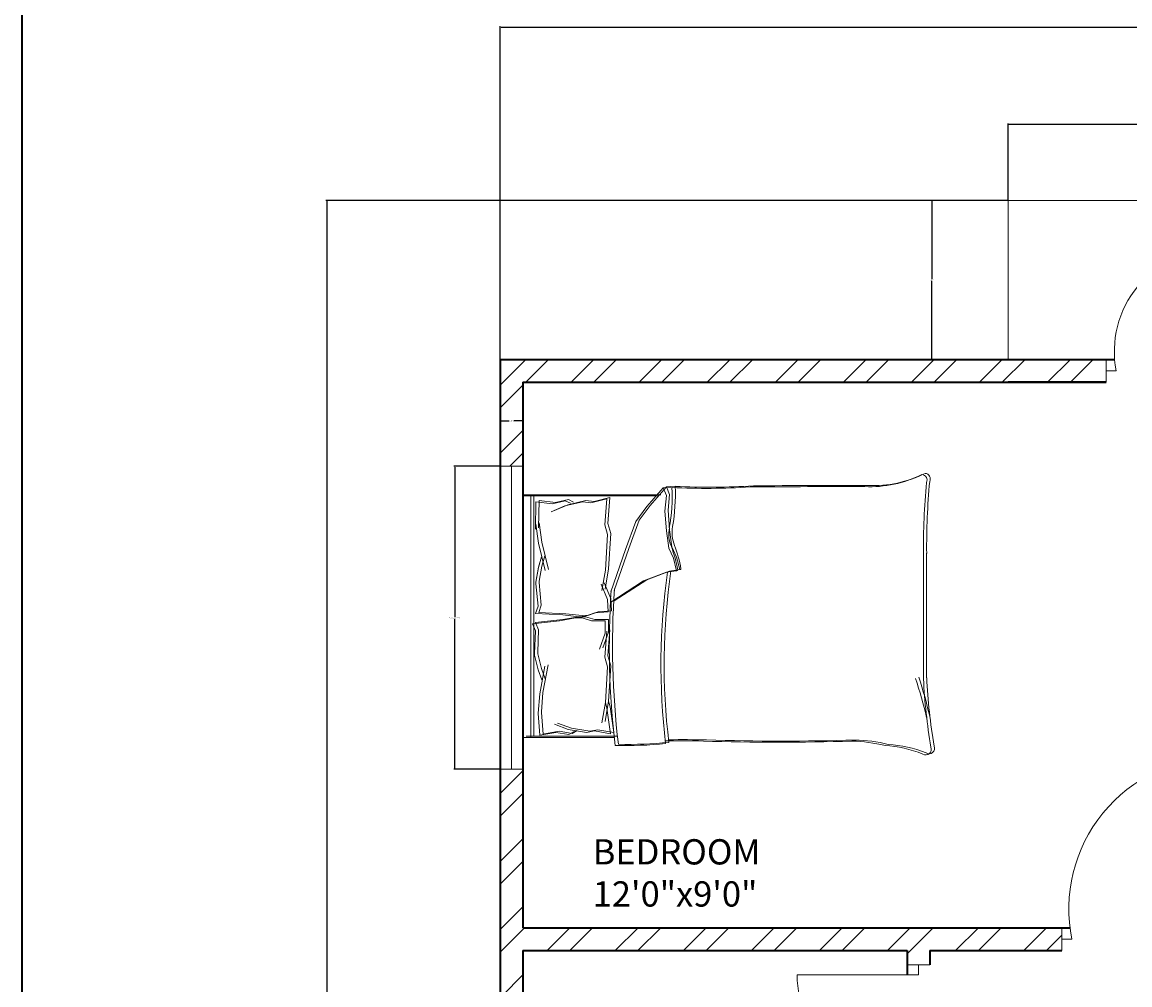
# Model space of a CAD drawing. Units: inches. Extents: x 2165 to 3042, y 1626 to 2968.
# Tile 3 of 11: x 2192 to 2411, y 2208 to 2399. Entities that reach past the tile are written whole.
import ezdxf

# ---------------------------------------------------------------- set-up
doc = ezdxf.new("R2010")
doc.units = ezdxf.units.IN
for name, color, linetype, lineweight in [('A-ANNO-DIMS', 2, 'Continuous', 18), ('A-AREA-IDEN', 7, 'Continuous', 18), ('A-DOOR', 3, 'Continuous', 18), ('A-FLOR-BALC', 7, 'Continuous', 18), ('A-FURN', 8, 'Continuous', 13), ('A-GLAZ', 4, 'Continuous', 18), ('A-WALL', 7, 'Continuous', 35), ('A-WALL-PATT', 252, 'Continuous', 13)]:
    doc.layers.add(name, color=color, linetype=linetype, lineweight=lineweight)
doc.styles.get("Standard").update_dxf_attribs({"font": 'arial.ttf'})
doc.dimstyles.get("Standard").update_dxf_attribs({"dimtxt": 0.18, "dimasz": 0.18, "dimexe": 0.18, "dimexo": 0.0625, "dimgap": 0.09, "dimtad": 0, "dimtih": 1, "dimtoh": 1, "dimdec": 4, "dimzin": 0, "dimdsep": 46, "dimtxsty": 'Standard', "dimcen": 0.09, "dimadec": 0, "dimazin": 0, "dimtfac": 1, "dimtdec": 4, "dimtofl": 0, "dimtmove": 0, "dimatfit": 3, "dimfxl": 1, "dimtolj": 1, "dimtzin": 0, "dimarcsym": 0})

# ---------------------------------------------------------------- blocks, each defined once
blk = doc.blocks.new('BED-DOUBLE')
for p, q in [((27.75, 52.87), (24.5, 49.16)), ((27.75, 52.87), (24.5, 49.16)), ((28.39, 53.1), (25.14, 49.39)), ((28.39, 53.1), (25.14, 49.39)), ((29.49, 52.95), (27.75, 52.87, 3.87)), ((29.49, 52.95), (27.75, 52.87, 3.87)), ((28.37, 51.33), (27.75, 52.87)), ((28.37, 51.33), (27.75, 52.87)), ((30.13, 53.18), (28.39, 53.1, 3.87)), ((30.13, 53.18), (28.39, 53.1, 3.87)), ((29, 51.56), (28.39, 53.1)), ((29, 51.56), (28.39, 53.1)), ((0, 51.27), (0, 51.49)), ((0, 51.49), (0.64, 51.49)), ((0, 51.27), (26.61, 51.27)), ((0, 51.27), (26.61, 51.27)), ((0, 51.27), (0, 3.48)), ((0.64, 51.49), (27.25, 51.49)), ((0.64, 51.49), (27.25, 51.49)), ((1.53, 3.48), (1.53, 51.27)), ((1.53, 3.47), (1.53, 51.27)), ((2.17, 3.7), (2.17, 51.49)), ((2.17, 3.7), (2.17, 51.49)), ((6.41, 49.96), (8.98, 50.56)), ((6.41, 49.96), (8.98, 50.56)), ((8.98, 50.56), (10.02, 50.04)), ((8.98, 50.56), (10.02, 50.04)), ((16.57, 50.7), (13.43, 49.92)), ((16.57, 50.7), (13.43, 49.92)), ((17.21, 50.93), (14.07, 50.15)), ((17.21, 50.93), (14.07, 50.15)), ((16.17, 45.57), (16.57, 50.7)), ((16.17, 45.57), (16.57, 50.7)), ((16.81, 45.79), (17.21, 50.93)), ((16.81, 45.79), (17.21, 50.93)), ((28.06, 48.23), (28.37, 51.33)), ((28.06, 48.23), (28.37, 51.33)), ((28.7, 48.46), (29, 51.56)), ((28.7, 48.46), (29, 51.56)), ((2.56, 50.11), (2.46, 44.71)), ((2.56, 50.11), (2.46, 44.71)), ((2.56, 50.11), (5.77, 49.73)), ((2.56, 50.11), (5.77, 49.73)), ((3.2, 50.34), (3.1, 44.94)), ((3.2, 50.34), (3.1, 44.94)), ((3.2, 50.34), (6.41, 49.96)), ((3.2, 50.34), (6.41, 49.96)), ((8.26, 49.31), (5.58, 48.13)), ((8.26, 49.31), (5.58, 48.13)), ((5.77, 49.73), (8.34, 50.33)), ((5.77, 49.73), (8.34, 50.33)), ((8.9, 49.54), (6.22, 48.36)), ((8.9, 49.54), (6.22, 48.36)), ((11.83, 50.11), (8.26, 49.31)), ((11.83, 50.11), (8.26, 49.31)), ((8.34, 50.33), (9.38, 49.81)), ((8.34, 50.33), (9.38, 49.81)), ((12.47, 50.34), (8.9, 49.54)), ((12.47, 50.34), (8.9, 49.54)), ((13.43, 49.92), (11.83, 50.11)), ((13.43, 49.92), (11.83, 50.11)), ((14.07, 50.15), (12.47, 50.34)), ((14.07, 50.15), (12.47, 50.34)), ((24.5, 49.16), (22.33, 46.22)), ((24.5, 49.16), (22.33, 46.22)), ((25.14, 49.39), (22.97, 46.45)), ((25.14, 49.39), (22.97, 46.45)), ((28.37, 44.36), (28.06, 48.23)), ((28.37, 44.36), (28.06, 48.23)), ((29, 44.59), (28.7, 48.46)), ((29, 44.59), (28.7, 48.46)), ((22.33, 46.22), (20.32, 40.64)), ((22.33, 46.22), (20.32, 40.64)), ((22.97, 46.45), (20.96, 40.87)), ((22.97, 46.45), (20.96, 40.87)), ((2.46, 44.71), (2.54, 45.71)), ((2.46, 44.71), (2.54, 45.71)), ((2.54, 45.71), (3.07, 41.91)), ((2.54, 45.71), (3.07, 41.91)), ((3.1, 44.94), (3.18, 45.94)), ((3.1, 44.94), (3.18, 45.94)), ((3.18, 45.94), (3.71, 42.14)), ((3.18, 45.94), (3.71, 42.14)), ((16.73, 43.61), (16.17, 45.57)), ((16.73, 43.61), (16.17, 45.57)), ((17.37, 43.83), (16.81, 45.79)), ((17.37, 43.83), (16.81, 45.79)), ((28.83, 40.95), (28.37, 44.36)), ((28.83, 40.95), (28.37, 44.36)), ((29.47, 41.18), (29, 44.59)), ((29.47, 41.18), (29, 44.59)), ((3.07, 41.91), (4.42, 36.5)), ((3.07, 41.91), (4.42, 36.49)), ((3.71, 42.14), (5.06, 36.72)), ((3.71, 42.14), (5.06, 36.72)), ((16.3, 36.6), (16.73, 43.61)), ((16.3, 36.6), (16.73, 43.61)), ((16.93, 36.82), (17.37, 43.83)), ((16.93, 36.82), (17.37, 43.83)), ((20.32, 40.64), (17.38, 32.31)), ((20.32, 40.64), (17.38, 32.31)), ((20.96, 40.87), (18.02, 32.53)), ((20.96, 40.87), (18.02, 32.53)), ((29.76, 38.94), (28.83, 40.95)), ((29.76, 38.94), (28.83, 40.95)), ((30.4, 39.17), (29.47, 41.18)), ((30.4, 39.17), (29.47, 41.18)), ((79.25, 15.06), (79.25, 39.68)), ((79.25, 15.06), (79.25, 39.68)), ((79.88, 15.29), (79.88, 39.91)), ((79.88, 15.29), (79.88, 39.91)), ((3.67, 39.2), (3.08, 37.14)), ((3.67, 39.2), (3.08, 37.13)), ((3.72, 37.36), (3.18, 34.43)), ((3.72, 37.36), (3.18, 34.43)), ((4.31, 39.43), (3.72, 37.36)), ((4.31, 39.43), (3.72, 37.36)), ((30.38, 36.46), (29.76, 38.94)), ((30.38, 36.46), (29.76, 38.94)), ((31.02, 36.69), (30.4, 39.17)), ((31.02, 36.69), (30.4, 39.17)), ((3.08, 37.14), (2.54, 34.2)), ((3.08, 37.13), (2.54, 34.2)), ((15.63, 32.56), (16.3, 36.6)), ((15.63, 32.56), (16.3, 36.6)), ((16.27, 32.79), (16.93, 36.82)), ((16.27, 32.79), (16.93, 36.82)), ((23.88, 34.45), (28.37, 36.15)), ((23.88, 34.45), (28.37, 36.15)), ((24.52, 34.68), (29, 36.38)), ((24.52, 34.68), (29, 36.38)), ((28.37, 36.15), (30.38, 36.46)), ((28.37, 36.15), (30.38, 36.46)), ((29, 36.38), (31.02, 36.69)), ((29, 36.38), (31.02, 36.69)), ((2.54, 34.2), (2.56, 33.88)), ((2.54, 34.2), (2.56, 33.88)), ((2.56, 33.88), (2.98, 29.46)), ((2.56, 33.88), (2.98, 29.46)), ((3.18, 34.43), (3.2, 34.11)), ((3.18, 34.43), (3.2, 34.11)), ((3.2, 34.11), (3.62, 29.68)), ((3.2, 34.11), (3.62, 29.68)), ((16.74, 30.75), (15.46, 33.82)), ((16.74, 30.75), (15.46, 33.82)), ((17.38, 30.98), (16.09, 34.05)), ((17.38, 30.98), (16.09, 34.05)), ((17.38, 30.26), (23.88, 34.45)), ((17.38, 30.26), (23.88, 34.45)), ((18.02, 30.49), (24.52, 34.68)), ((18.02, 30.49), (24.52, 34.68)), ((16.89, 28.3), (16.74, 30.75)), ((16.89, 28.3), (16.74, 30.75)), ((17.53, 28.53), (17.38, 30.98)), ((17.53, 28.53), (17.38, 30.98)), ((2.98, 29.46), (2.49, 27.98)), ((2.98, 29.46), (2.49, 27.98)), ((3.62, 29.68), (3.13, 28.21)), ((3.62, 29.68), (3.13, 28.21)), ((14.86, 28.36), (17.53, 28.53)), ((14.86, 28.36), (17.53, 28.53)), ((1.87, 25.98), (7.22, 26.56)), ((1.87, 25.98), (7.22, 26.56)), ((2.49, 27.98), (7.87, 27.73)), ((2.49, 27.98), (7.87, 27.73)), ((2.51, 26.21), (7.86, 26.79)), ((2.51, 26.21), (7.86, 26.79)), ((3.13, 28.21), (8.51, 27.96)), ((3.13, 28.21), (8.51, 27.96)), ((7.22, 26.56), (10.4, 27.14)), ((7.22, 26.56), (10.4, 27.14)), ((7.86, 26.79), (11.04, 27.37)), ((7.86, 26.79), (11.04, 27.37)), ((7.87, 27.73), (11.08, 27.35)), ((7.87, 27.73), (11.08, 27.35)), ((8.51, 27.96), (11.72, 27.58)), ((8.51, 27.96), (11.72, 27.58)), ((10.4, 27.14), (11.7, 27.14)), ((10.4, 27.14), (11.7, 27.14)), ((11.04, 27.37), (12.34, 27.37)), ((11.04, 27.37), (12.34, 27.37)), ((11.08, 27.35), (12.38, 27.44)), ((11.08, 27.35), (12.38, 27.44)), ((11.7, 27.14), (13.58, 26.56)), ((11.7, 27.14), (13.58, 26.56)), ((11.72, 27.58), (13.02, 27.66)), ((11.72, 27.58), (13.02, 27.66)), ((12.34, 27.37), (14.22, 26.79)), ((12.34, 27.37), (14.22, 26.79)), ((12.38, 27.44), (14.22, 28.13)), ((12.38, 27.44), (14.22, 28.13)), ((13.02, 27.66), (14.86, 28.36)), ((13.02, 27.66), (14.86, 28.36)), ((13.58, 26.56), (16.26, 26.56)), ((13.58, 26.56), (16.26, 26.56)), ((14.22, 28.13), (16.89, 28.3)), ((14.22, 28.13), (16.89, 28.3)), ((14.22, 26.79), (16.9, 26.79)), ((14.22, 26.79), (16.9, 26.79)), ((16.26, 26.56), (16.26, 24.1)), ((16.26, 26.56), (16.26, 24.1)), ((16.9, 26.79), (16.9, 24.33)), ((16.9, 26.79), (16.9, 24.33)), ((2.45, 24.54), (1.87, 25.98)), ((2.45, 24.54), (1.87, 25.98)), ((2.3, 20.09), (2.45, 24.54)), ((2.3, 20.09), (2.45, 24.54)), ((3.09, 24.77), (2.51, 26.21)), ((3.09, 24.77), (2.51, 26.21)), ((2.94, 20.32), (3.09, 24.77)), ((2.94, 20.32), (3.09, 24.77)), ((16.9, 24.33), (15.81, 21.19)), ((16.9, 24.33), (15.81, 21.19)), ((16.17, 19.38), (16.57, 24.52)), ((16.17, 19.38), (16.57, 24.52)), ((16.81, 19.61), (17.21, 24.74)), ((16.81, 19.61), (17.21, 24.74)), ((16.26, 24.1), (15.17, 20.96)), ((16.26, 24.1), (15.17, 20.96)), ((2.3, 19.77), (2.3, 20.09)), ((2.3, 19.77), (2.3, 20.09)), ((3.03, 16.88), (2.3, 19.77)), ((3.03, 16.88), (2.3, 19.77)), ((2.94, 20), (2.94, 20.32)), ((2.94, 20), (2.94, 20.32)), ((3.67, 17.11), (2.94, 20)), ((3.67, 17.11), (2.94, 20)), ((3.32, 12.11), (4.33, 17.6)), ((3.32, 12.11), (4.33, 17.6)), ((3.96, 12.34), (4.97, 17.83)), ((3.96, 12.34), (4.97, 17.83)), ((16.73, 17.42), (16.17, 19.38)), ((16.73, 17.42), (16.17, 19.38)), ((17.37, 17.65), (16.81, 19.61)), ((17.37, 17.65), (16.81, 19.61)), ((16.93, 10.64), (17.37, 17.65)), ((16.93, 10.64), (17.37, 17.65)), ((3.75, 14.85), (3.03, 16.88)), ((3.75, 14.85), (3.03, 16.88)), ((4.39, 15.08), (3.67, 17.11)), ((4.39, 15.08), (3.67, 17.11)), ((16.3, 10.41), (16.73, 17.42)), ((16.3, 10.41), (16.73, 17.42)), ((3.03, 8.28), (3.32, 12.11)), ((3.03, 8.28), (3.32, 12.11)), ((3.67, 8.51), (3.96, 12.34)), ((3.67, 8.51), (3.96, 12.34)), ((15.63, 6.38), (16.3, 10.41)), ((15.63, 6.38), (16.3, 10.41)), ((16.27, 6.61), (16.93, 10.64)), ((16.27, 6.61), (16.93, 10.64)), ((16.3, 10.41), (16.62, 9.28)), ((16.3, 10.41), (16.62, 9.28)), ((16.62, 9.28), (17.34, 4.18)), ((16.62, 9.28), (17.34, 4.18)), ((16.93, 10.64), (17.26, 9.51)), ((16.93, 10.64), (17.26, 9.51)), ((17.26, 9.51), (17.98, 4.41)), ((17.26, 9.51), (17.98, 4.41)), ((3.01, 8.18), (3.03, 8.28)), ((3.01, 8.18), (3.03, 8.28)), ((3.34, 3.9), (3.01, 8.18)), ((3.34, 3.9), (3.01, 8.18)), ((3.65, 8.41), (3.67, 8.51)), ((3.65, 8.41), (3.67, 8.51)), ((3.98, 4.13), (3.65, 8.41)), ((3.98, 4.13), (3.65, 8.41)), ((3.32, 3.89), (6.5, 4.47)), ((3.32, 3.89), (6.5, 4.47)), ((3.96, 4.12), (7.14, 4.7)), ((3.96, 4.12), (7.14, 4.7)), ((8.96, 5.05), (6.21, 6.06)), ((8.96, 5.05), (6.21, 6.06)), ((6.5, 4.47), (9.1, 4.04)), ((6.5, 4.47), (9.1, 4.04)), ((9.59, 5.28), (6.85, 6.29)), ((9.59, 5.28), (6.85, 6.29)), ((7.14, 4.7), (9.74, 4.27)), ((7.14, 4.7), (9.74, 4.27)), ((12.57, 4.47), (8.96, 5.05)), ((12.57, 4.47), (8.96, 5.05)), ((9.1, 4.04), (10.11, 4.62)), ((9.1, 4.04), (10.11, 4.62)), ((13.21, 4.7), (9.59, 5.28)), ((13.21, 4.7), (9.59, 5.28)), ((9.74, 4.27), (10.75, 4.85)), ((9.74, 4.27), (10.75, 4.85)), ((14.16, 4.76), (12.57, 4.47)), ((14.16, 4.76), (12.57, 4.47)), ((14.8, 4.99), (13.21, 4.7)), ((14.8, 4.99), (13.21, 4.7)), ((17.34, 4.18), (14.16, 4.76)), ((17.34, 4.18), (14.16, 4.76)), ((17.98, 4.41), (14.8, 4.99)), ((17.98, 4.41), (14.8, 4.99)), ((18.11, 3.48), (0, 3.48)), ((18.11, 3.47), (0, 3.47)), ((18.75, 3.7), (0.64, 3.7)), ((18.75, 3.7), (0.64, 3.7))]:
    blk.add_line(p, q)
for centre, radius, start, end in [((68.67, 76.16), 23.07, 267.4714, 296.4681), ((68.67, 76.16), 23.07, 267.4714, 296.4681), ((69.31, 76.39), 23.07, 267.4714, 296.4681), ((69.31, 76.39), 23.07, 267.4714, 296.4681), ((78.87, 54.41), 1.1, 332.6588, 86.02), ((78.87, 54.41), 1.1, 332.6588, 86.02), ((79.51, 54.64), 1.1, 332.6588, 86.02), ((79.51, 54.64), 1.1, 332.6588, 86.02), ((-6.66, 51.33), 36.18, 349.8763, 2.5657), ((-6.66, 51.33), 36.18, 349.8763, 2.5657), ((36.32, 182.27), 129.5, 266.9791, 273.8365), ((36.32, 182.27), 129.5, 266.9791, 273.8365), ((-6.02, 51.56), 36.18, 349.8763, 2.5657), ((-6.02, 51.56), 36.18, 349.8763, 2.5657), ((36.95, 182.49), 129.5, 266.9791, 273.8365), ((36.95, 182.49), 129.5, 266.9791, 273.8365), ((67.82, -4508.74), 4561.86, 90.00217, 90.28689), ((67.82, -4508.74), 4561.86, 90.00217, 90.28689), ((68.46, -4508.52), 4561.86, 90.00217, 90.28689), ((68.46, -4508.52), 4561.86, 90.00217, 90.28689), ((212.28, 41.15), 133.04, 174.4998, 180.6351), ((212.28, 41.15), 133.04, 174.4998, 180.6351), ((212.92, 41.38), 133.04, 174.4998, 180.6351), ((212.92, 41.38), 133.04, 174.4998, 180.6351), ((35.07, 43.74), 6.22, 168.6608, 203.7384), ((35.07, 43.74), 6.22, 168.6608, 203.7384), ((35.71, 43.97), 6.22, 168.6608, 203.7384), ((35.71, 43.97), 6.22, 168.6608, 203.7384), ((1.48, 31.15), 29.65, 10.6617, 19.8806), ((1.48, 31.15), 29.65, 10.6617, 19.8806), ((2.12, 31.38), 29.65, 10.6617, 19.8806), ((2.12, 31.38), 29.65, 10.6617, 19.8806), ((156.32, 17.76), 129.02, 171.7845, 186.9006), ((156.32, 17.76), 129.02, 171.7845, 186.9006), ((156.96, 17.98), 129.02, 171.7845, 186.9006), ((156.96, 17.98), 129.02, 171.7845, 186.9006), ((30.44, 36.64), 0.185, 250.2464, 1.1377), ((30.44, 36.64), 0.185, 250.2464, 1.1377), ((31.08, 36.86), 0.185, 250.2464, 1.1377), ((31.08, 36.86), 0.185, 250.2464, 1.1377), ((182.05, 21.36), 164.97, 176.0865, 186.7821), ((182.05, 21.36), 164.97, 176.0865, 186.7821), ((182.69, 21.59), 164.97, 176.0865, 186.7821), ((182.69, 21.59), 164.97, 176.0865, 186.7821), ((-23.07, -16.99), 106.46, 13.3832, 17.7053), ((-23.07, -16.99), 106.46, 13.3832, 17.7053), ((-23.71, -17.22), 106.46, 13.3832, 17.7053), ((-23.71, -17.22), 106.46, 13.3832, 17.7053), ((200.84, 21.43), 121.76, 182.9958, 189.4091), ((200.84, 21.43), 121.76, 182.9958, 189.4091), ((201.48, 21.66), 121.76, 182.9958, 189.4091), ((201.48, 21.65), 121.76, 182.9958, 189.4091), ((20.1, 85.16), 83.31, 268.7218, 275.604), ((20.1, 85.16), 83.31, 268.7218, 275.604), ((20.74, 85.39), 83.31, 268.7218, 275.604), ((20.74, 85.39), 83.31, 268.7218, 275.604), ((31.17, -167.31), 170.11, 88.4762, 91.0082), ((31.17, -167.31), 170.11, 88.4762, 91.0082), ((31.81, -167.08), 170.11, 88.4762, 91.0082), ((31.81, -167.08), 170.11, 88.4762, 91.0082), ((50.61, 484.82), 482.31, 268.2277, 271.7185), ((50.61, 484.82), 482.31, 268.2277, 271.7185), ((51.25, 485.05), 482.31, 268.2277, 271.7185), ((51.25, 485.05), 482.31, 268.2277, 271.7185), ((64.52, -26.9), 29.63, 76.0648, 88.9113), ((64.52, -26.9), 29.63, 76.0648, 88.9113), ((65.15, -26.67), 29.63, 76.0648, 88.9113), ((65.15, -26.67), 29.63, 76.0648, 88.9113), ((70.28, -21.66), 23.56, 67.9751, 86.652), ((70.28, -21.66), 23.56, 67.9751, 86.652), ((70.92, -21.43), 23.56, 67.9751, 86.652), ((70.92, -21.43), 23.56, 67.9751, 86.652), ((79.72, 1.09), 1.09, 236.1736, 23.4781), ((79.72, 1.09), 1.09, 236.1736, 23.4781), ((80.36, 1.32), 1.09, 236.1736, 23.4781), ((80.36, 1.32), 1.09, 236.1736, 23.4781)]:
    blk.add_arc(centre, radius, start, end)
blk = doc.blocks.new('BALCONY-RAIL-PLAN')
for p, q in [((0, 31.5), (0, 0)), ((100.5, 31.5), (100.5, 0)), ((100.5, 0), (0, 0))]:
    blk.add_line(p, q)
blk = doc.blocks.new('WIN-60-A')
for p, q in [((4.5, 60), (0, 60)), ((0, 60), (2.25, 60)), ((2.25, 60), (2.25, 0)), ((2.25, 0), (0, 0)), ((0, 0), (4.5, 0))]:
    blk.add_line(p, q)
blk = doc.blocks.new('*D24')
at = {"layer": 'A-ANNO-DIMS', "color": 0, "lineweight": -2, "transparency": 16777216}
for p, q in [((2387.1, 2363.64), (2387.1, 2378.83)), ((2387.28, 2378.65), (2435.81, 2378.65)), ((2487.42, 2378.65), (2438.9, 2378.65)), ((2487.6, 2363.64), (2487.6, 2378.83))]:
    blk.add_line(p, q, dxfattribs=at)
at = {"layer": 'A-ANNO-DIMS', "color": 0, "transparency": 16777216}
for points in [[(2387.28, 2378.68), (2387.28, 2378.62), (2387.1, 2378.65)], [(2487.42, 2378.68), (2487.42, 2378.62), (2487.6, 2378.65)]]:
    blk.add_solid(points, dxfattribs=at)
at = {"layer": 'Defpoints', "color": 0, "transparency": 16777216}
for p in [(2387.1, 2378.65), (2387.1, 2363.58), (2487.6, 2363.58)]:
    blk.add_point(p, dxfattribs=at)
at = {"layer": 'A-ANNO-DIMS', "color": 0, "transparency": 16777216, "insert": (2437.35, 2378.65), "char_height": 0.18, "attachment_point": 5}
blk.add_mtext('\\A1;BALCONY RAIL 101 TYP.', dxfattribs=at)
blk = doc.blocks.new('*D25')
at = {"layer": 'A-ANNO-DIMS', "color": 0, "lineweight": -2, "transparency": 16777216}
for p, q in [((2387.04, 2363.58), (2371.85, 2363.58)), ((2372.03, 2363.4), (2372.03, 2348.01)), ((2372.03, 2332.26), (2372.03, 2347.65)), ((2387.04, 2332.08), (2371.85, 2332.08))]:
    blk.add_line(p, q, dxfattribs=at)
at = {"layer": 'A-ANNO-DIMS', "color": 0, "transparency": 16777216}
for points in [[(2372, 2363.4), (2372.06, 2363.4), (2372.03, 2363.58)], [(2372, 2332.26), (2372.06, 2332.26), (2372.03, 2332.08)]]:
    blk.add_solid(points, dxfattribs=at)
at = {"layer": 'Defpoints', "color": 0, "transparency": 16777216}
for p in [(2387.1, 2363.58), (2372.03, 2332.08), (2387.1, 2332.08)]:
    blk.add_point(p, dxfattribs=at)
at = {"layer": 'A-ANNO-DIMS', "color": 0, "transparency": 16777216, "insert": (2372.03, 2347.83), "char_height": 0.18, "attachment_point": 5}
blk.add_mtext('\\A1;32 TYP.', dxfattribs=at)
blk = doc.blocks.new('*D34')
at = {"layer": 'A-ANNO-DIMS', "color": 0, "lineweight": -2, "transparency": 16777216}
for p, q in [((2286.54, 2310.97), (2277.42, 2310.97)), ((2277.6, 2310.79), (2277.6, 2281.15)), ((2277.6, 2251.15), (2277.6, 2280.78)), ((2286.54, 2250.97), (2277.42, 2250.97))]:
    blk.add_line(p, q, dxfattribs=at)
at = {"layer": 'A-ANNO-DIMS', "color": 0, "transparency": 16777216}
for points in [[(2277.57, 2310.79), (2277.63, 2310.79), (2277.6, 2310.97)], [(2277.57, 2251.15), (2277.63, 2251.15), (2277.6, 2250.97)]]:
    blk.add_solid(points, dxfattribs=at)
at = {"layer": 'Defpoints', "color": 0, "transparency": 16777216}
for p in [(2277.6, 2310.97), (2286.6, 2310.97), (2286.6, 2250.97)]:
    blk.add_point(p, dxfattribs=at)
at = {"layer": 'A-ANNO-DIMS', "color": 0, "transparency": 16777216, "insert": (2277.6, 2280.97), "char_height": 0.18, "attachment_point": 5}
blk.add_mtext('\\A1;WINDOW A 60 TYP.', dxfattribs=at)
blk = doc.blocks.new('*D35')
at = {"layer": 'A-ANNO-DIMS', "color": 0, "lineweight": -2, "transparency": 16777216}
for p, q in [((2286.6, 2311.03), (2286.6, 2320.15)), ((2286.78, 2319.97), (2288.4, 2319.97)), ((2290.92, 2319.97), (2289.31, 2319.97)), ((2291.1, 2311.03), (2291.1, 2320.15))]:
    blk.add_line(p, q, dxfattribs=at)
at = {"layer": 'A-ANNO-DIMS', "color": 0, "transparency": 16777216}
for points in [[(2286.78, 2320), (2286.78, 2319.94), (2286.6, 2319.97)], [(2290.92, 2320), (2290.92, 2319.94), (2291.1, 2319.97)]]:
    blk.add_solid(points, dxfattribs=at)
at = {"layer": 'Defpoints', "color": 0, "transparency": 16777216}
for p in [(2291.1, 2319.97), (2286.6, 2310.97), (2291.1, 2310.97)]:
    blk.add_point(p, dxfattribs=at)
at = {"layer": 'A-ANNO-DIMS', "color": 0, "transparency": 16777216, "insert": (2288.85, 2319.97), "char_height": 0.18, "attachment_point": 5}
blk.add_mtext('\\A1;5 TYP.', dxfattribs=at)
blk = doc.blocks.new('*D50')
at = {"layer": 'A-ANNO-DIMS', "color": 0, "lineweight": -2, "transparency": 16777216}
for p, q in [((2286.6, 2332.14), (2286.6, 2398.06)), ((2885.1, 2332.14), (2885.1, 2398.06)), ((2286.78, 2397.88), (2585.46, 2397.88)), ((2884.92, 2397.88), (2586.25, 2397.88))]:
    blk.add_line(p, q, dxfattribs=at)
at = {"layer": 'A-ANNO-DIMS', "color": 0, "transparency": 16777216}
for points in [[(2286.78, 2397.91), (2286.78, 2397.85), (2286.6, 2397.88)], [(2884.92, 2397.91), (2884.92, 2397.85), (2885.1, 2397.88)]]:
    blk.add_solid(points, dxfattribs=at)
at = {"layer": 'Defpoints', "color": 0, "transparency": 16777216}
for p in [(2885.1, 2397.88), (2286.6, 2332.08), (2885.1, 2332.08)]:
    blk.add_point(p, dxfattribs=at)
at = {"layer": 'A-ANNO-DIMS', "color": 0, "transparency": 16777216, "insert": (2585.85, 2397.88), "char_height": 0.18, "attachment_point": 5}
blk.add_mtext('\\A1;598.5', dxfattribs=at)
blk = doc.blocks.new('*D51')
at = {"layer": 'A-ANNO-DIMS', "color": 0, "lineweight": -2, "transparency": 16777216}
for p, q in [((2387.04, 2363.58), (2252.12, 2363.58)), ((2252.3, 2363.4), (2252.3, 2082.76)), ((2252.3, 1801.76), (2252.3, 2082.4)), ((2535.54, 1801.58), (2252.12, 1801.58))]:
    blk.add_line(p, q, dxfattribs=at)
at = {"layer": 'A-ANNO-DIMS', "color": 0, "transparency": 16777216}
for points in [[(2252.27, 2363.4), (2252.33, 2363.4), (2252.3, 2363.58)], [(2252.27, 1801.76), (2252.33, 1801.76), (2252.3, 1801.58)]]:
    blk.add_solid(points, dxfattribs=at)
at = {"layer": 'Defpoints', "color": 0, "transparency": 16777216}
for p in [(2252.3, 2363.58), (2387.1, 2363.58), (2535.6, 1801.58)]:
    blk.add_point(p, dxfattribs=at)
at = {"layer": 'A-ANNO-DIMS', "color": 0, "transparency": 16777216, "insert": (2252.3, 2082.58), "char_height": 0.18, "attachment_point": 5}
blk.add_mtext('\\A1;562', dxfattribs=at)

msp = doc.modelspace()

# ---------------------------------------------------------------- hatches: boundary and pattern name
at = {"layer": 'A-WALL-PATT'}
h = msp.add_hatch(dxfattribs=at)
h.set_pattern_fill('ANSI32', color=256)
h.paths.add_polyline_path([(2406.4931, 2332.0783), (2286.6045, 2332.0783), (2286.6045, 2310.967), (2288.8545, 2310.967), (2291.1045, 2310.967), (2291.1045, 2327.5783), (2406.4931, 2327.5783), (2406.4931, 2329.8283)])
h.paths.add_polyline_path([(2439.6045, 2327.5783), (2444.9584, 2327.5783), (2444.9584, 2332.0783), (2430.2901, 2332.0783), (2430.2901, 2329.8283), (2430.2901, 2327.5783), (2435.1045, 2327.5783), (2435.1045, 2219.5783), (2431.0902, 2219.5783), (2431.0902, 2215.0783), (2435.1045, 2215.0783), (2444.1108, 2215.0783), (2444.1108, 2217.3283), (2444.1108, 2219.5783), (2439.6045, 2219.5783)])
h.paths.add_polyline_path([(2497.5418, 2329.8283), (2497.5418, 2332.0783), (2470.1978, 2332.0783), (2470.1978, 2327.5783), (2497.5418, 2327.5783)])
h.paths.add_polyline_path([(2617.9543, 2332.0783), (2557.5418, 2332.0783), (2557.5418, 2327.5783), (2583.6045, 2327.5783), (2583.6045, 2219.5783), (2474.0523, 2219.5783), (2474.0523, 2215.0783), (2583.6045, 2215.0783), (2583.6045, 2107.0783), (2579.3609, 2107.0783), (2579.3609, 2102.5783), (2588.1045, 2102.5783), (2593.5283, 2102.5783), (2593.5283, 2104.8283), (2593.5283, 2107.0783), (2588.1045, 2107.0783), (2588.1045, 2215.0783), (2691.2325, 2215.0783), (2691.2325, 2217.3283), (2691.2325, 2219.5783), (2588.1045, 2219.5783), (2588.1045, 2327.5783), (2617.9543, 2327.5783)])
h.paths.add_polyline_path([(2702.4444, 2329.8283), (2702.4444, 2332.0783), (2677.9543, 2332.0783), (2677.9543, 2327.5783), (2702.4444, 2327.5783)])
h.paths.add_polyline_path([(2736.6045, 2327.5783), (2742.5161, 2327.5783), (2742.5161, 2329.8283), (2742.5161, 2332.0783), (2727.7639, 2332.0783), (2727.7639, 2329.8283), (2727.7639, 2327.5783), (2732.1045, 2327.5783), (2732.1045, 2219.5783), (2726.4404, 2219.5783), (2726.4404, 2215.0783), (2732.1045, 2215.0783), (2742.7291, 2215.0783), (2742.7291, 2217.3283), (2742.7291, 2219.5783), (2736.6045, 2219.5783)])
h.paths.add_polyline_path([(2885.1045, 2332.0783), (2768.4887, 2332.0783), (2768.4887, 2327.5783), (2784.6045, 2327.5783), (2880.6045, 2327.5783), (2880.6045, 2310.967), (2885.1045, 2310.967)])
h.paths.add_polyline_path([(2885.1045, 2250.967), (2880.6045, 2250.967), (2880.6045, 2219.5783), (2776.5755, 2219.5783), (2776.5755, 2215.0783), (2788.1045, 2215.0783), (2788.1045, 2209.8634), (2790.3545, 2209.8634), (2792.6045, 2209.8634), (2792.6045, 2215.0783), (2880.6045, 2215.0783), (2880.6045, 2139.0783), (2871.2037, 2139.0783), (2871.2037, 2134.5783), (2885.1045, 2134.5783)])
h.paths.add_polyline_path([(2545.013, 2107.0783), (2474.0523, 2107.0783), (2291.1045, 2107.0783), (2291.1045, 2102.5783), (2535.6045, 2102.5783), (2535.6045, 2096.8046), (2537.8545, 2096.8046), (2540.1045, 2096.8046), (2540.1045, 2102.5783), (2545.013, 2102.5783), (2545.013, 2104.8283)])
h.paths.add_polyline_path([(2397.7297, 2217.3283), (2397.7297, 2219.5783), (2291.1045, 2219.5783), (2291.1045, 2250.967), (2286.6045, 2250.967), (2286.6045, 2206.1346), (2288.8545, 2206.1346), (2291.1045, 2206.1346), (2291.1045, 2215.0783), (2367.1045, 2215.0783), (2367.1045, 2212.2868), (2371.6045, 2212.2868), (2371.6045, 2215.0783), (2397.7297, 2215.0783)])
h.paths.add_polyline_path([(2291.1045, 1978.5783), (2367.1045, 1978.5783), (2371.6045, 1978.5783), (2373.2641, 1978.5783), (2374.4883, 1978.5783), (2374.4883, 1980.8283), (2374.4883, 1983.0783), (2371.6045, 1983.0783), (2371.6045, 1986.964), (2369.9051, 1986.964), (2369.3545, 1986.964), (2367.1045, 1986.964), (2367.1045, 1983.0783), (2291.1045, 1983.0783), (2291.1045, 2001.1808), (2286.6045, 2001.1808), (2286.6045, 1947.0203), (2288.8545, 1947.0203), (2291.1045, 1947.0203)])
h.paths.add_polyline_path([(2291.1045, 1887.0203), (2286.6045, 1887.0203), (2286.6045, 1842.0783), (2381.2561, 1842.0783), (2381.2561, 1844.3283), (2381.2561, 1846.5783), (2363.1045, 1846.5783), (2291.1045, 1846.5783)])
h.paths.add_polyline_path([(2415.6045, 1978.5783), (2421.1681, 1978.5783), (2421.1681, 1983.0783), (2415.6045, 1983.0783), (2406.5227, 1983.0783), (2406.5227, 1980.8283), (2406.5227, 1978.5783), (2411.1045, 1978.5783), (2411.1045, 1846.5783), (2406.7549, 1846.5783), (2406.7549, 1842.0783), (2419.2885, 1842.0783), (2419.2885, 1844.3283), (2419.2885, 1846.5783), (2415.6045, 1846.5783)])
h.paths.add_polyline_path([(2586.6045, 1982.779), (2586.6045, 1991.5911), (2582.1045, 1991.5911), (2582.1045, 1982.779), (2540.1045, 1982.779), (2540.1045, 2036.779), (2582.1045, 2036.779), (2582.1045, 2027.6051), (2586.6045, 2027.6051), (2586.6045, 2041.279), (2582.1045, 2041.279), (2540.1045, 2041.279), (2540.1045, 2063.9064), (2537.8545, 2063.9064), (2535.6045, 2063.9064), (2535.6045, 1983.0783), (2455.068, 1983.0783), (2455.068, 1978.5783), (2535.6045, 1978.5783), (2535.6045, 1846.5783), (2522.622, 1846.5783), (2522.622, 1842.0783), (2535.6045, 1842.0783), (2535.6045, 1806.0783), (2535.6045, 1801.5783), (2556.726, 1801.5783), (2556.726, 1803.8283), (2556.726, 1806.0783), (2540.1045, 1806.0783), (2540.1045, 1842.0783), (2540.1045, 1846.5783), (2540.1045, 1978.279), (2586.6045, 1978.279)])
h.paths.add_polyline_path([(2636.1045, 1978.5783), (2717.6642, 1978.5783), (2717.6642, 1980.8283), (2717.6642, 1983.0783), (2636.1045, 1983.0783), (2636.1045, 2063.9064), (2633.8545, 2063.9064), (2631.6045, 2063.9064), (2631.6045, 1846.5783), (2631.6045, 1842.0783), (2631.6045, 1806.0783), (2604.726, 1806.0783), (2604.726, 1801.5783), (2636.1045, 1801.5783), (2636.1045, 1842.0783), (2644.3411, 1842.0783), (2644.3411, 1844.3283), (2644.3411, 1846.5783), (2636.1045, 1846.5783)])
h.paths.add_polyline_path([(2760.6045, 1978.5783), (2764.9931, 1978.5783), (2764.9931, 1983.0783), (2750.4727, 1983.0783), (2750.4727, 1980.8283), (2750.4727, 1978.5783), (2756.1045, 1978.5783), (2756.1045, 1846.5783), (2749.4543, 1846.5783), (2749.4543, 1842.0783), (2765.1894, 1842.0783), (2765.1894, 1846.5783), (2760.6045, 1846.5783)])
h.paths.add_polyline_path([(2880.6045, 1983.0783), (2804.6045, 1983.0783), (2804.6045, 1988.3825), (2802.3545, 1988.3825), (2800.1045, 1988.3825), (2800.1045, 1983.0783), (2800.1045, 1978.5783), (2880.6045, 1978.5783)])
h.paths.add_polyline_path([(2885.1045, 2075.5783), (2871.2037, 2075.5783), (2871.2037, 2071.0783), (2880.6045, 2071.0783), (2880.6045, 1948.8144), (2885.1045, 1948.8144)])
h.paths.add_polyline_path([(2885.1045, 1888.8144), (2880.6045, 1888.8144), (2880.6045, 1846.5783), (2792.1167, 1846.5783), (2792.1167, 1842.0783), (2885.1045, 1842.0783)])
h.paths.add_polyline_path([(2724.4848, 1846.5783), (2708.1045, 1846.5783), (2692.3411, 1846.5783), (2692.3411, 1842.0783), (2724.4848, 1842.0783), (2724.4848, 1844.3283)])
h.paths.add_polyline_path([(2474.622, 1844.4672), (2474.622, 1846.5783), (2444.7417, 1846.5783), (2444.7417, 1842.0783), (2474.622, 1842.0783)])

# ---------------------------------------------------------------- linework, layer by layer
at = {"layer": 'A-DOOR'}
for p, q in [((2406.4931, 2332.0783), (2406.4931, 2327.5783)), ((2406.4931, 2327.5783), (2406.4931, 2329.8283)), ((2406.4931, 2329.8283), (2408.4931, 2329.8283)), ((2397.7297, 2219.5783), (2397.7297, 2215.0783)), ((2397.7297, 2215.0783), (2397.7297, 2217.3283)), ((2397.7297, 2217.3283), (2399.7297, 2217.3283)), ((2367.1045, 2212.2868), (2371.6045, 2212.2868)), ((2371.6045, 2212.2868), (2369.3545, 2212.2868)), ((2369.3545, 2212.2868), (2369.3545, 2210.2868)), ((2369.3545, 2210.2868), (2345.3545, 2210.2868))]:
    msp.add_line(p, q, dxfattribs=at)
for centre, radius, start, end in [((2428.2901, 2333.6633), 20.165, 90, 190.963229), ((2429.0902, 2223.3556), 29.9727, 90, 191.600845), ((2363.5239, 2210.2868), 18.1694, 180, 288.717485)]:
    msp.add_arc(centre, radius, start, end, dxfattribs=at)
at = {"layer": 'A-WALL'}
for p, q in [((2286.6045, 2332.0783), (2408.1874, 2332.0783)), ((2286.6045, 2332.0783), (2408.1874, 2332.0783)), ((2286.6045, 2332.0783), (2286.6045, 1842.0783)), ((2291.1045, 2327.5783), (2406.4931, 2327.5783)), ((2291.1045, 2327.5783), (2291.1045, 2219.5783)), ((2406.4931, 2327.5783), (2387.1045, 2327.5783)), ((2291.1045, 2219.5783), (2399.3564, 2219.5783)), ((2291.1045, 2215.0783), (2367.1045, 2215.0783)), ((2291.1045, 2215.0783), (2291.1045, 2167.0783)), ((2367.1045, 2215.0783), (2367.1045, 2210.2868)), ((2371.6045, 2215.0783), (2371.6045, 2212.2868)), ((2371.6045, 2215.0783), (2397.7297, 2215.0783))]:
    msp.add_line(p, q, dxfattribs=at)
msp.add_lwpolyline([(2191.9961, 2967.8547), (3042.3708, 2967.8547), (3042.3708, 1626.3264), (2191.9961, 1626.3264)], close=True, dxfattribs=at)

# ---------------------------------------------------------------- block references
at = {"layer": 'A-FLOR-BALC', "rotation": 180}
msp.add_blockref('BALCONY-RAIL-PLAN', (2487.6049, 2363.5786), dxfattribs=at)
at = {"layer": 'A-FURN'}
msp.add_blockref('BED-DOUBLE', (2291.104, 2253.813), dxfattribs=at)
at = {"layer": 'A-GLAZ'}
msp.add_blockref('WIN-60-A', (2286.604, 2250.967), dxfattribs=at)

# ---------------------------------------------------------------- texts
at = {"layer": 'A-AREA-IDEN', "insert": (2304.905, 2237.1329), "char_height": 5, "attachment_point": 1}
msp.add_mtext_dynamic_manual_height_columns('BEDROOM\\P12\'0"x9\'0"', width=137.914823, gutter_width=12.5, heights=[0], dxfattribs=at)

# ---------------------------------------------------------------- dimensions: what is measured, and where the dimension line sits
at = {"layer": 'A-ANNO-DIMS'}
dim = msp.add_linear_dim(base=(2885.1045, 2397.8783), p1=(2286.6045, 2332.0783), p2=(2885.1045, 2332.0783), dimstyle='Standard', override={"dimdec": 1, "dimlfac": 1, "dimrnd": 0, "dimzin": 0, "dimdsep": 46, "dimlunit": 2}, dxfattribs=at)
dim.commit()
dim.dimension.update_dxf_attribs({"geometry": '*D50', "text_midpoint": (2585.8545, 2397.8783)})
for base, p1, p2, angle, text, picture, middle in [((2387.1044518572, 2378.6533076613), (2487.6044518572, 2363.5783076613), (2387.1044518572, 2363.5783076613), 180, 'BALCONY RAIL <> TYP.', '*D24', (2437.3544518572, 2378.6533076613)), ((2372.0294518572, 2332.0783076613), (2387.1044518572, 2363.5783076613), (2387.1044518572, 2332.0783076613), 270, '<> TYP.', '*D25', (2372.0294518572, 2347.8283076613)), ((2277.6045, 2310.967), (2286.6045, 2250.967), (2286.6045, 2310.967), 90, 'WINDOW A <> TYP.', '*D34', (2277.6045, 2280.967))]:
    dim = msp.add_linear_dim(base=base, p1=p1, p2=p2, angle=angle, text=text, dimstyle='Standard', override={"dimdec": 0, "dimlfac": 1, "dimrnd": 0, "dimzin": 0, "dimdsep": 46, "dimlunit": 2}, dxfattribs=at)
    dim.commit()
    dim.dimension.update_dxf_attribs({"geometry": picture, "text_midpoint": middle})
dim = msp.add_linear_dim(base=(2252.3045, 2363.5783), p1=(2535.6045, 1801.5783), p2=(2387.1045, 2363.5783), angle=90, dimstyle='Standard', override={"dimdec": 0, "dimlfac": 1, "dimrnd": 0, "dimzin": 0, "dimdsep": 46, "dimlunit": 2}, dxfattribs=at)
dim.commit()
dim.dimension.update_dxf_attribs({"geometry": '*D51', "text_midpoint": (2252.3045, 2082.5783)})
dim = msp.add_linear_dim(base=(2291.1044518572, 2319.9669825207), p1=(2286.6044518572, 2310.9669825207), p2=(2291.1044518572, 2310.9669825207), text='<> TYP.', dimstyle='Standard', override={"dimdec": 0, "dimlfac": 1, "dimrnd": 0, "dimzin": 0, "dimdsep": 46, "dimlunit": 2}, dxfattribs=at)
dim.commit()
dim.dimension.update_dxf_attribs({"geometry": '*D35', "text_midpoint": (2288.8544518572, 2319.9669825207)})

doc.saveas('drawing.dxf')
